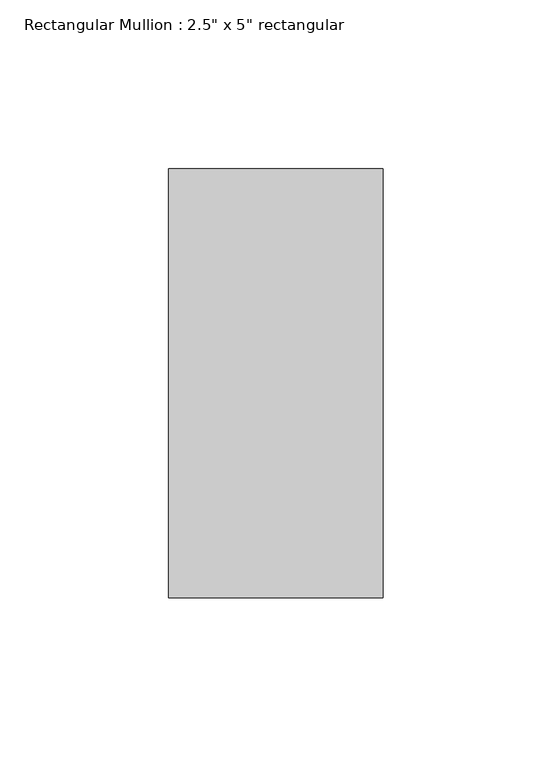
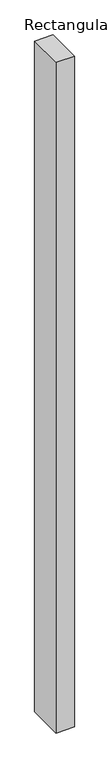
"""IFC4 building model written with IfcOpenShell, lengths in millimetres: member geometry."""

from ifc_helpers import new_model, si_unit, frame, origin, place, context, project, spatial, polyline, outline, extrude, source, transform, mapped, element, save


def member_d6a8c742(model_context):
    return source(origin(), model_context, "Body", "SweptSolid", [
        extrude(outline(polyline([(0.0, 63.5), (0.0, -63.5), (-63.5, -63.5), (-63.5, 63.5), (0.0, 63.5)])), frame((0.0, 0.0, -2446.4380434), z_axis=(0.0, 0.0, 1.0), x_axis=(1.0, 0.0, 0.0)), (0.0, 0.0, 1.0), 2446.4380434),
    ])


if __name__ == "__main__":
    model = new_model("IFC4")
    model_context = context("Model", 3, world=origin())
    ifc_project = project(units=[si_unit("LENGTHUNIT", "METRE", prefix="MILLI")], contexts=[model_context])
    site = spatial("IfcSite", under=ifc_project)
    building = spatial("IfcBuilding", under=site)
    placement = place(None, origin())
    member_shape = member_d6a8c742(model_context)
    element("IfcMember", 1, ObjectType="Rectangular Mullion : 2.5\" x 5\" rectangular", at=placement, inside=building, context=model_context, shape_type="MappedRepresentation", body=[
        mapped(member_shape, transform((0.0, 0.0, 0.0), x_axis=(1.0, 0.0, 0.0), y_axis=(0.0, 1.0, 0.0), z_axis=(0.0, 0.0, 1.0))),
    ])
    save(model, "model.ifc")

# Revit data of these elements
# Type "Rectangular Mullion : 2.5\" x 5\" rectangular"
#   built-in parameter 1007304 = 0.416667 (stored number, unit not read)
#   built-in parameter 1007301 = 0.104167 (stored number, unit not read)
#   built-in parameter 1007300 = 0.104167 (stored number, unit not read)
# Element 1 (IfcMember, "Rectangular Mullion : 2.5\" x 5\" rectangular")
#   Materials on its faces: "Aluminum"
# Materials
#   "Aluminum": class "Metal", colour RGB 247 247 247, transparency 0, Description = "Aluminum 6061", Cost = 0
